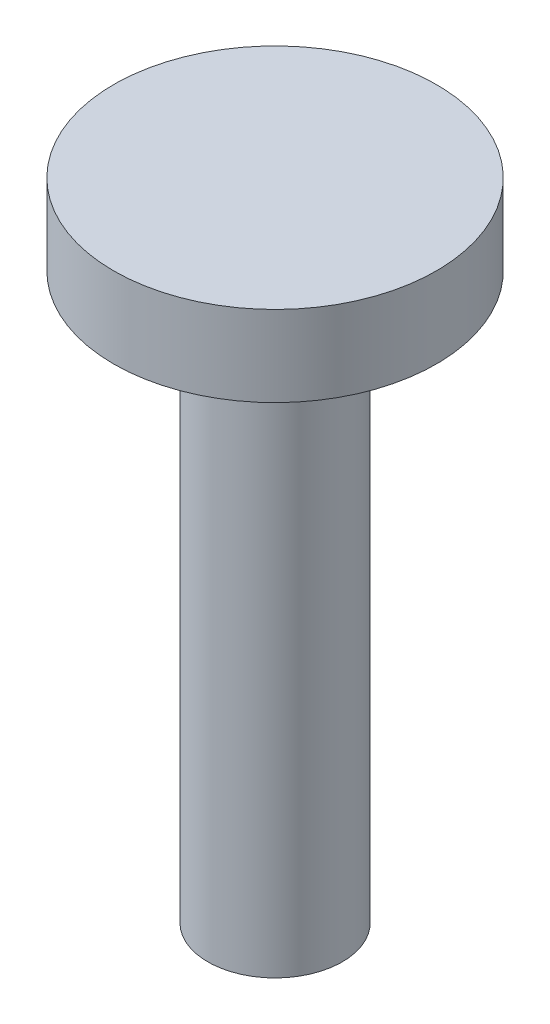
SolidWorks part; units mm, degrees
material "Plain Carbon Steel"
ref_plane "Front Plane" through (0, 0, 0) normal (0, 0, 1) x (1, 0, 0)
ref_plane "Top Plane" through (0, 0, 0) normal (0, 1, 0) x (1, 0, 0)
ref_plane "Right Plane" through (0, 0, 0) normal (1, 0, 0) x (0, 0, -1)
sketch "Shank Profile Ø5" plane through (0, 0, 0) normal (0, 1, 0) x (1, 0, 0)
  circle A0 centre (0, 0) radius 2.5
  dimension "D1" = 5
extrude "Shank Ø5x21" add sketch "Shank Profile Ø5" along normal mid plane 21
sketch "Head Profile Ø12" plane through (0, 10.5, 0) normal (0, 1, 0) x (1, 0, 0)
  circle A0 centre (0, 0) radius 6
  dimension "D1" = 12
extrude "Head Ø12x3" add sketch "Head Profile Ø12" along normal blind 3
